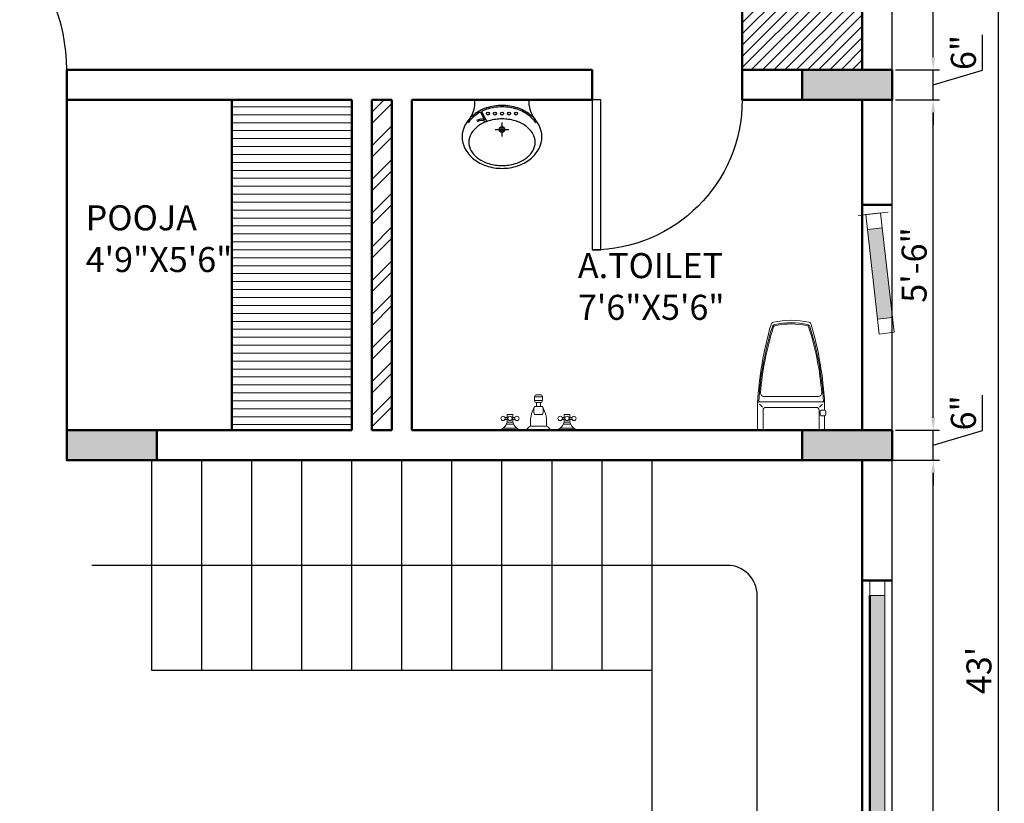
# Model space of a CAD drawing. Units: inches. Extents: x 3064 to 19385, y 846 to 15425.
# Tile 59 of 108: x 6210 to 6407, y 1703 to 1860. Entities that reach past the tile are written whole.
import ezdxf

# ---------------------------------------------------------------- set-up
doc = ezdxf.new("R2010")
doc.units = ezdxf.units.IN
for name, color, linetype, lineweight in [('A-ANNO-DIMS', 2, 'Continuous', 18), ('A-AREA-IDEN', 3, 'Continuous', 18), ('A-COLS', 1, 'Continuous', 35), ('A-DOOR', 3, 'Continuous', 25), ('A-FLOR-FIXT', 9, 'Continuous', 18), ('A-FLOR-STRS', 2, 'Continuous', 25), ('A-FURN-PATT', 252, 'Continuous', 13), ('A-GLAZ', 4, 'Continuous', 18), ('A-WALL', 7, 'Continuous', 50), ('C-PROP', 6, 'Continuous', 25)]:
    doc.layers.add(name, color=color, linetype=linetype, lineweight=lineweight)
doc.layers.add('THIET-BI', color=21, linetype='Continuous')
doc.styles.get("Standard").update_dxf_attribs({"font": 'arial.ttf'})
doc.dimstyles.new('ISO-25', dxfattribs={"dimtxt": 9, "dimasz": 2.5, "dimexe": 1.25, "dimexo": 0.625, "dimtad": 1, "dimdec": 1, "dimlunit": 3, "dimtxsty": 'Standard', "dimcen": 2.5, "dimadec": 0, "dimazin": 0, "dimtfac": 1, "dimtdec": 1, "dimtmove": 0, "dimatfit": 3, "dimfxl": 1, "dimarcsym": 0})

# ---------------------------------------------------------------- blocks, each defined once
blk = doc.blocks.new('*U3')
for p, q in [((0, 0), (0, -6)), ((36, 0), (36, -6))]:
    blk.add_line(p, q)
blk.add_lwpolyline([(0, 0), (0, 36), (1.75, 36), (1.75, 0)], close=True)
blk.add_arc((0, 0), 36, 0, 90)
blk = doc.blocks.new('*U4')
for p, q in [((0, 0), (0, -6)), ((30, 0), (30, -6))]:
    blk.add_line(p, q)
blk.add_lwpolyline([(0, 0), (0, 30), (1.75, 30), (1.75, 0)], close=True)
blk.add_arc((0, 0), 30, 0, 90)
blk = doc.blocks.new('A$C430D11A0')
at = {"layer": 'THIET-BI'}
for p, q in [((90, 445), (90, 485)), ((475, 485), (90, 485)), ((475, 483), (90, 483)), ((475, 445), (475, 485)), ((129.4, 398.5), (158.2, 344.4)), ((138.3, 403), (176, 332.4)), ((282.5, 226.2), (282.5, 324.8)), ((233.4, 275.5), (331.9, 275.5))]:
    blk.add_line(p, q, dxfattribs=at)
for points in [[(565, 222.5, 0.121635), (544.7, 304.8, 0.10526), (482.3, 379.8, 0.088175), (393.4, 427.4, 0.079002), (282.5, 445, 0.079002), (171.6, 427.4, 0.088175), (82.7, 379.8, 0.10526), (20.3, 304.8, 0.121635), (0, 222.5, 0.121635), (20.3, 140.2, 0.10526), (82.7, 65.2, 0.088175), (171.6, 17.6, 0.079002), (282.5, 0, 0.079002), (393.4, 17.6, 0.088175), (482.3, 65.2, 0.10526), (544.7, 140.2, 0.121635)], [(517.5, 185, 0.134042), (501.2, 244.9, 0.106817), (448.7, 301.7, 0.082468), (375.6, 336.7, 0.070874), (282.5, 350, 0.070874), (189.4, 336.7, 0.082468), (116.3, 301.7, 0.106817), (63.8, 244.9, 0.134042), (47.5, 185, 0.134042), (63.8, 125.1, 0.106817), (116.3, 68.3, 0.082468), (189.4, 33.3, 0.070874), (282.5, 20, 0.070874), (375.6, 33.3, 0.082468), (448.7, 68.3, 0.106817), (501.2, 125.1, 0.134042)]]:
    blk.add_lwpolyline(points, format="xyb", close=True, dxfattribs=at)
for points in [[(522.9, 321.6, 0.07708), (476.1, 372, 0.088175), (390.3, 417.9, 0.079002), (282.5, 435, 0.079002), (174.7, 417.9, 0.035427), (138.3, 403, 0.07708)], [(129.4, 398.5, 0.043566), (88.9, 372, 0.07708), (42.1, 321.6, 0.041486)]]:
    blk.add_lwpolyline(points, format="xyb", dxfattribs=at)
for centre, radius in [((182.5, 388.2), 10.5), ((232.5, 388.2), 10.5), ((282.5, 388.2), 10.5), ((332.5, 388.2), 10.5), ((382.5, 388.2), 10.5), ((282.5, 275.5), 20), ((282.5, 275.5), 15)]:
    blk.add_circle(centre, radius, dxfattribs=at)
for centre, radius, start, end in [((-103.8, 468.9), 195.3, 320.8253, 352.95569), ((668.8, 468.9), 195.3, 187.04431, 219.1747), ((136.4, 285.4), 62.9, 69.64296, 123.47738), ((136.4, 285.4), 52.9, 55.24551, 123.47738)]:
    blk.add_arc(centre, radius, start, end, dxfattribs=at)
blk = doc.blocks.new('WC-P05')
for p, q in [((-202.4, 531.6), (-202.4, 439.1)), ((-192.4, 541.6), (262.6, 541.6)), ((-163.4, 541.6), (-163.4, 400.6)), ((233.6, 541.6), (233.6, 400.6)), ((272.6, 531.6), (272.6, 351.6)), ((-210.4, 430.1), (-210.4, 409.1)), ((-201.4, 439.1), (-180.4, 439.1)), ((-171.4, 430.1), (-171.4, 409.1)), ((-202.4, 400.1), (-202.4, 351.6)), ((-201.4, 400.1), (-180.4, 400.1)), ((-166.9, 378.6), (-188.2, 357.3)), ((-143.4, 380.6), (213.6, 380.6)), ((237.1, 378.6), (258.4, 357.3)), ((-192.4, 341.6), (262.6, 341.6)), ((-159.3, 302.6), (229.5, 302.6))]:
    blk.add_line(p, q)
blk.add_lwpolyline([(-90.9, -221.9, 0.114547), (161, -222, 0.114547)], format="xyb")
for centre, radius, start, end in [((-192.4, 531.6), 10, 90, 180), ((262.6, 531.6), 10, 0, 90), ((-201.4, 430.1), 9, 90, 180), ((-180.4, 430.1), 9, 0, 90), ((-201.4, 409.1), 9, 180, 270), ((2308.9, 492.3), 2515.2, 183.20675, 196.12415), ((-192.4, 351.6), 10, 180, 270), ((-180.4, 409.1), 9, 270, 0), ((-143.4, 400.6), 20, 180, 270), ((-2238.7, 492.3), 2515.2, 343.87268, 356.79325), ((213.6, 400.6), 20, 270, 0), ((262.6, 351.6), 10, 270, 0), ((1906, 447.2), 2102.6, 182.87428, 197.65536), ((-159.3, 280.1), 22.5, 90, 184.62462), ((-1835.8, 447.2), 2102.6, 342.34464, 357.12572), ((229.5, 280.1), 22.5, 355.37538, 90), ((1905.9, 447.2), 2094.5, 184.62454, 197.52765), ((-1835.8, 447.2), 2094.6, 342.46396, 355.37538), ((-85.8, -199.9), 22.5, 196.12415, 256.89941), ((-76.1, -183.7), 22.5, 197.65536, 257.50587), ((-69.9, -176.8), 22.5, 197.52765, 258.10049), ((35.1, 318), 536.4, 257.50587, 282.49413), ((35.7, 324.3), 534.7, 258.10049, 281.73735), ((139.9, -177.1), 22.5, 281.73735, 342.46396), ((146.2, -183.7), 22.5, 282.49413, 342.34464), ((155.9, -200.1), 22.5, 283.03778, 343.87268)]:
    blk.add_arc(centre, radius, start, end)
blk = doc.blocks.new('Faucet - Bathroom front')
for p, q in [((-0.5, 4.25), (0.5, 4.25)), ((0.5, 3.75), (-0.5, 3.75)), ((-0.5, 3), (0.5, 3)), ((-0.25, 3), (-0.25, 3.5)), ((0.25, 3.5), (0.25, 3)), ((-4, 1.625), (-4.25, 1.625)), ((-4, 1.375), (-4.25, 1.375)), ((-3.25, 1.625), (-3, 1.625)), ((-3.25, 1.375), (-3, 1.375)), ((0.5, 2), (-0.5, 2)), ((3.25, 1.625), (3, 1.625)), ((3.25, 1.375), (3, 1.375)), ((4, 1.625), (4.25, 1.625)), ((4, 1.375), (4.25, 1.375)), ((-5, 0), (-2.25, 0)), ((-4.5087, 0.25), (-2.7408, 0.25)), ((-3.1442, 0.75), (-4.0979, 0.75)), ((-1.5, 0), (1.5, 0)), ((-1, 0.5), (1, 0.5)), ((2.25, 0), (5, 0)), ((2.7413, 0.25), (4.5092, 0.25)), ((4.1058, 0.75), (3.1521, 0.75))]:
    blk.add_line(p, q)
for points in [[(-0.5, 3.75), (-0.5, 4.25)], [(-0.25, 4.5), (0.25, 4.5)], [(0.5, 4.25), (0.5, 3.75)], [(0.25, 3.5), (-0.25, 3.5)]]:
    blk.add_lwpolyline(points)
for points in [[(-4, 1), (-4, 2), (-3.25, 2), (-3.25, 1)], [(3.25, 1), (3.25, 2), (4, 2), (4, 1)]]:
    blk.add_lwpolyline(points, close=True)
for centre in [(-4.5, 1.5), (-3.625, 1.5), (-2.75, 1.5), (2.75, 1.5), (3.625, 1.5), (4.5, 1.5)]:
    blk.add_circle(centre, 0.2795)
for centre, radius, start, end in [((-0.2575, 4.2575), 0.2426, 88.22243, 181.7776), ((0.2575, 4.2575), 0.2426, 358.2224, 91.77757), ((3, 1), 4.0311, 150.2551, 187.125), ((0.6413, 2.5), 1.246, 156.3417, 203.6583), ((-0.2575, 3.7425), 0.2426, 178.2224, 271.7776), ((0.2575, 3.7425), 0.2426, 268.2224, 1.777565), ((-3, 1), 4.0311, 352.875, 29.74488), ((-0.6413, 2.5), 1.246, 336.3417, 23.65835), ((-5.375, 1.375), 1.4252, 285.2551, 344.7449), ((-1.875, 1.375), 1.4252, 195.2551, 254.7449), ((-0.7962, -0.2038), 0.7327, 106.1502, 163.8498), ((0.7962, -0.2038), 0.7327, 16.1502, 73.84979), ((1.875, 1.375), 1.4252, 285.2551, 344.7449), ((5.375, 1.375), 1.4252, 195.2551, 254.7449)]:
    blk.add_arc(centre, radius, start, end)
blk = doc.blocks.new('*D350')
at = {"layer": 'A-ANNO-DIMS', "color": 0, "lineweight": -2, "transparency": 16777216}
for p, q in [((6379.12, 1771.99), (6393.94, 1771.99)), ((6392.69, 1576.49), (6392.69, 1769.49)), ((6379.12, 1573.99), (6393.94, 1573.99))]:
    blk.add_line(p, q, dxfattribs=at)
at = {"layer": 'A-ANNO-DIMS', "color": 0, "transparency": 16777216}
for points in [[(6392.27, 1769.49), (6393.1, 1769.49), (6392.69, 1771.99)], [(6392.27, 1576.49), (6393.1, 1576.49), (6392.69, 1573.99)]]:
    blk.add_solid(points, dxfattribs=at)
at = {"layer": 'Defpoints', "color": 0, "transparency": 16777216}
for p in [(6378.49, 1771.99), (6392.69, 1771.99), (6378.49, 1573.99)]:
    blk.add_point(p, dxfattribs=at)
at = {"layer": 'A-ANNO-DIMS', "color": 0, "transparency": 16777216, "insert": (6389.51, 1672.99), "char_height": 5, "attachment_point": 5, "rotation": 90}
blk.add_mtext('16\'-6"', dxfattribs=at)
blk = doc.blocks.new('*D351')
at = {"layer": 'A-ANNO-DIMS', "color": 0, "lineweight": -2, "transparency": 16777216}
for p, q in [((6402.53, 1777.94), (6402.53, 1784.97)), ((6392.69, 1780.49), (6392.69, 1782.99)), ((6385.12, 1777.99), (6393.94, 1777.99)), ((6392.69, 1771.99), (6392.69, 1777.99)), ((6392.69, 1771.99), (6392.69, 1777.99)), ((6392.69, 1774.99), (6402.53, 1777.94)), ((6379.12, 1771.99), (6393.94, 1771.99)), ((6392.69, 1769.49), (6392.69, 1766.99))]:
    blk.add_line(p, q, dxfattribs=at)
at = {"layer": 'A-ANNO-DIMS', "color": 0, "transparency": 16777216}
for points in [[(6392.27, 1780.49), (6393.1, 1780.49), (6392.69, 1777.99)], [(6392.27, 1769.49), (6393.1, 1769.49), (6392.69, 1771.99)]]:
    blk.add_solid(points, dxfattribs=at)
at = {"layer": 'Defpoints', "color": 0, "transparency": 16777216}
for p in [(6384.49, 1777.99), (6392.69, 1777.99), (6378.49, 1771.99)]:
    blk.add_point(p, dxfattribs=at)
at = {"layer": 'A-ANNO-DIMS', "color": 0, "transparency": 16777216, "insert": (6399.35, 1781.45), "char_height": 5, "attachment_point": 5, "rotation": 90}
blk.add_mtext('6"', dxfattribs=at)
blk = doc.blocks.new('*D352')
at = {"layer": 'A-ANNO-DIMS', "color": 0, "lineweight": -2, "transparency": 16777216}
for p, q in [((6385.12, 1843.99), (6393.94, 1843.99)), ((6392.69, 1780.49), (6392.69, 1841.49)), ((6385.12, 1777.99), (6393.94, 1777.99))]:
    blk.add_line(p, q, dxfattribs=at)
at = {"layer": 'A-ANNO-DIMS', "color": 0, "transparency": 16777216}
for points in [[(6392.27, 1841.49), (6393.1, 1841.49), (6392.69, 1843.99)], [(6392.27, 1780.49), (6393.1, 1780.49), (6392.69, 1777.99)]]:
    blk.add_solid(points, dxfattribs=at)
at = {"layer": 'Defpoints', "color": 0, "transparency": 16777216}
for p in [(6384.49, 1843.99), (6392.69, 1843.99), (6384.49, 1777.99)]:
    blk.add_point(p, dxfattribs=at)
at = {"layer": 'A-ANNO-DIMS', "color": 0, "transparency": 16777216, "insert": (6389.51, 1810.99), "char_height": 5, "attachment_point": 5, "rotation": 90}
blk.add_mtext('5\'-6"', dxfattribs=at)
blk = doc.blocks.new('*D353')
at = {"layer": 'A-ANNO-DIMS', "color": 0, "lineweight": -2, "transparency": 16777216}
for p, q in [((6402.53, 1849.94), (6402.53, 1856.97)), ((6392.69, 1852.49), (6392.69, 1854.99)), ((6385.12, 1849.99), (6393.94, 1849.99)), ((6392.69, 1843.99), (6392.69, 1849.99)), ((6392.69, 1843.99), (6392.69, 1849.99)), ((6392.69, 1846.99), (6402.53, 1849.94)), ((6385.12, 1843.99), (6393.94, 1843.99)), ((6392.69, 1841.49), (6392.69, 1838.99))]:
    blk.add_line(p, q, dxfattribs=at)
at = {"layer": 'A-ANNO-DIMS', "color": 0, "transparency": 16777216}
for points in [[(6392.27, 1852.49), (6393.1, 1852.49), (6392.69, 1849.99)], [(6392.27, 1841.49), (6393.1, 1841.49), (6392.69, 1843.99)]]:
    blk.add_solid(points, dxfattribs=at)
at = {"layer": 'Defpoints', "color": 0, "transparency": 16777216}
for p in [(6384.49, 1849.99), (6392.69, 1849.99), (6384.49, 1843.99)]:
    blk.add_point(p, dxfattribs=at)
at = {"layer": 'A-ANNO-DIMS', "color": 0, "transparency": 16777216, "insert": (6399.35, 1853.45), "char_height": 5, "attachment_point": 5, "rotation": 90}
blk.add_mtext('6"', dxfattribs=at)
blk = doc.blocks.new('*D375')
at = {"layer": 'A-ANNO-DIMS', "color": 0, "lineweight": -2, "transparency": 16777216}
for p, q in [((6379.12, 1981.99), (6393.94, 1981.99)), ((6392.69, 1852.49), (6392.69, 1979.49)), ((6385.12, 1849.99), (6393.94, 1849.99))]:
    blk.add_line(p, q, dxfattribs=at)
at = {"layer": 'A-ANNO-DIMS', "color": 0, "transparency": 16777216}
for points in [[(6392.27, 1979.49), (6393.1, 1979.49), (6392.69, 1981.99)], [(6392.27, 1852.49), (6393.1, 1852.49), (6392.69, 1849.99)]]:
    blk.add_solid(points, dxfattribs=at)
at = {"layer": 'Defpoints', "color": 0, "transparency": 16777216}
for p in [(6378.49, 1981.99), (6392.69, 1981.99), (6384.49, 1849.99)]:
    blk.add_point(p, dxfattribs=at)
at = {"layer": 'A-ANNO-DIMS', "color": 0, "transparency": 16777216, "insert": (6389.55, 1915.99), "char_height": 5, "attachment_point": 5, "rotation": 90}
blk.add_mtext("11'", dxfattribs=at)
blk = doc.blocks.new('*D377')
at = {"layer": 'A-ANNO-DIMS', "color": 0, "lineweight": -2, "transparency": 16777216}
for p, q in [((6385.12, 1987.99), (6406.89, 1987.99)), ((6405.64, 1985.49), (6405.64, 1474.49)), ((6385.12, 1471.99), (6406.89, 1471.99))]:
    blk.add_line(p, q, dxfattribs=at)
at = {"layer": 'A-ANNO-DIMS', "color": 0, "transparency": 16777216}
for points in [[(6405.22, 1985.49), (6406.05, 1985.49), (6405.64, 1987.99)], [(6405.22, 1474.49), (6406.05, 1474.49), (6405.64, 1471.99)]]:
    blk.add_solid(points, dxfattribs=at)
at = {"layer": 'Defpoints', "color": 0, "transparency": 16777216}
for p in [(6384.49, 1987.99), (6384.49, 1471.99), (6405.64, 1471.99)]:
    blk.add_point(p, dxfattribs=at)
at = {"layer": 'A-ANNO-DIMS', "color": 0, "transparency": 16777216, "insert": (6402.46, 1729.99), "char_height": 5, "attachment_point": 5, "rotation": 90}
blk.add_mtext("43'", dxfattribs=at)
blk = doc.blocks.new('WIN-1800-PAIR')
h = blk.add_hatch(color=256)
h.dxf.hatch_style = 1
h.paths.add_polyline_path([(0, 0), (3, 0), (3, 70.5), (0, 70.5)])
h.paths.add_polyline_path([(3, 144), (0, 144), (0, 73.5), (3, 73.5)])
blk.add_line((3, 144), (3, 73.5))
blk.add_lwpolyline([(3, 144), (0, 144), (0, 147), (3, 147)], close=True)
blk = doc.blocks.new('WIN-600-B')
h = blk.add_hatch(color=256)
h.dxf.hatch_style = 1
h.paths.add_polyline_path([(4.5, 21), (1.5, 21), (1.5, 3), (4.5, 3)])
for p, q in [((1.5, 21), (1.5, 3)), ((4.5, 21), (4.5, 3)), ((0, 0), (6, 0))]:
    blk.add_line(p, q)
for points in [[(4.5, 21), (1.5, 21), (1.5, 24), (4.5, 24)], [(4.5, 0), (1.5, 0), (1.5, 3), (4.5, 3)]]:
    blk.add_lwpolyline(points, close=True)

msp = doc.modelspace()

# ---------------------------------------------------------------- hatches: boundary and pattern name
at = {"layer": 'A-COLS'}
h = msp.add_hatch(color=256, dxfattribs=at)
h.dxf.hatch_style = 1
h.paths.add_polyline_path([(6384.49, 1843.99), (6384.49, 1849.99), (6366.49, 1849.99), (6366.49, 1843.99)])
h = msp.add_hatch(color=256, dxfattribs=at)
h.dxf.hatch_style = 1
h.paths.add_polyline_path([(6237.49, 1771.99), (6237.49, 1777.99), (6219.49, 1777.99), (6219.49, 1771.99)])
h = msp.add_hatch(color=256, dxfattribs=at)
h.dxf.hatch_style = 1
h.paths.add_polyline_path([(6384.49, 1771.99), (6384.49, 1777.99), (6366.49, 1777.99), (6366.49, 1771.99)])
at = {"layer": 'A-FURN-PATT'}
h = msp.add_hatch(dxfattribs=at)
h.set_pattern_fill('ANSI31', color=256, scale=0.5)
h.set_pattern_definition([(45, (726.825, 591.649), (-1.122532, 1.122532), [])])
h.paths.add_polyline_path([(6354.49, 1849.99), (6378.49, 1849.99), (6378.49, 1981.99), (6354.49, 1981.99)])
h = msp.add_hatch(dxfattribs=at)
h.set_pattern_fill('ANSI31', color=256, scale=0.5, angle=135)
h.set_pattern_definition([(180, (726.825, 591.649), (-1e-16, -1.5875), [])])
h.paths.add_polyline_path([(6252.49, 1777.99), (6276.49, 1777.99), (6276.49, 1843.99), (6252.49, 1843.99)])
h = msp.add_hatch(dxfattribs=at)
h.set_pattern_fill('ANSI32', color=256, scale=0.5)
h.set_pattern_definition([(45, (726.825, 591.649), (-3.367596, 3.367596), []), (45, (729.07, 591.649), (-3.367596, 3.367596), [])])
h.paths.add_polyline_path([(6280.49, 1777.99), (6284.49, 1777.99), (6284.49, 1843.99), (6280.49, 1843.99)])

# ---------------------------------------------------------------- linework, layer by layer
at = {"layer": 'A-FLOR-STRS'}
for p, q in [((6236.49, 1729.99), (6236.49, 1771.99)), ((6246.49, 1729.99), (6246.49, 1771.99)), ((6256.49, 1729.99), (6256.49, 1771.99)), ((6266.49, 1729.99), (6266.49, 1771.99)), ((6276.49, 1729.99), (6276.49, 1771.99)), ((6286.49, 1729.99), (6286.49, 1771.99)), ((6296.49, 1729.99), (6296.49, 1771.99)), ((6306.49, 1729.99), (6306.49, 1771.99)), ((6316.49, 1729.99), (6316.49, 1771.99)), ((6326.49, 1729.99), (6326.49, 1771.99)), ((6336.49, 1615.99), (6336.49, 1771.99)), ((6336.49, 1729.99), (6236.49, 1729.99))]:
    msp.add_line(p, q, dxfattribs=at)
msp.add_lwpolyline([(6243.98, 1594.99), (6351.49, 1594.99, 0.414214), (6357.49, 1600.99), (6357.49, 1744.99, 0.414214), (6351.49, 1750.99), (6224.49, 1750.99)], format="xyb", dxfattribs=at)
at = {"layer": 'A-WALL'}
for p, q in [((6354.49, 1843.99), (6354.49, 1981.99)), ((6378.49, 1849.99), (6378.49, 1981.99)), ((6324.49, 1849.99), (6219.49, 1849.99)), ((6219.49, 1849.99), (6219.49, 1771.99)), ((6324.49, 1843.99), (6324.49, 1849.99)), ((6378.49, 1849.99), (6354.49, 1849.99)), ((6276.49, 1843.99), (6219.49, 1843.99)), ((6252.49, 1843.99), (6252.49, 1777.99)), ((6276.49, 1843.99), (6276.49, 1777.99)), ((6284.49, 1843.99), (6280.49, 1843.99)), ((6280.49, 1843.99), (6280.49, 1777.99)), ((6284.49, 1777.99), (6284.49, 1843.99)), ((6288.49, 1777.99), (6288.49, 1843.99)), ((6324.49, 1843.99), (6288.49, 1843.99)), ((6378.49, 1843.99), (6354.49, 1843.99)), ((6378.49, 1777.99), (6378.49, 1843.99)), ((6378.49, 1822.99), (6384.49, 1822.99)), ((6276.49, 1777.99), (6219.49, 1777.99)), ((6284.49, 1777.99), (6280.49, 1777.99)), ((6378.49, 1777.99), (6288.49, 1777.99)), ((6378.49, 1771.99), (6219.49, 1771.99)), ((6378.49, 1573.99), (6378.49, 1771.99)), ((6384.49, 1747.99), (6378.49, 1747.99)), ((6379.99, 1744.99), (6379.99, 1674.49))]:
    msp.add_line(p, q, dxfattribs=at)
for points in [[(6384.49, 1849.99), (6366.49, 1849.99), (6366.49, 1843.99), (6384.49, 1843.99)], [(6237.49, 1777.99), (6219.49, 1777.99), (6219.49, 1771.99), (6237.49, 1771.99)], [(6384.49, 1777.99), (6366.49, 1777.99), (6366.49, 1771.99), (6384.49, 1771.99)]]:
    msp.add_lwpolyline(points, close=True, dxfattribs=at)
at = {"layer": 'C-PROP'}
msp.add_line((6384.49, 1471.99), (6384.49, 1987.99), dxfattribs=at)

# ---------------------------------------------------------------- block references
at = {"layer": 'A-DOOR'}
msp.add_blockref('*U3', (6183.49, 1849.99), dxfattribs=at)
at = {"layer": 'A-DOOR', "xscale": -1, "rotation": 180}
msp.add_blockref('*U4', (6324.49, 1843.99), dxfattribs=at)
at = {"layer": 'A-FLOR-FIXT'}
for name, p, xscale, yscale, zscale in [('A$C430D11A0', (6298.52, 1830.3), 0.0282220760332506, 0.0282220760332506, 0.0282220760332506), ('Faucet - Bathroom front', (6313.79, 1777.99), 1.573166238287219, 1.573166238287219, 1.573166238287219)]:
    msp.add_blockref(name, p, dxfattribs=dict(at, xscale=xscale, yscale=yscale, zscale=zscale))
at = {"layer": 'A-FLOR-FIXT', "xscale": 0.0282220760332506, "yscale": 0.0282220760332506, "zscale": 0.0282220760332506, "rotation": 180}
msp.add_blockref('WC-P05', (6365.27, 1793.28), dxfattribs=at)
at = {"layer": 'A-GLAZ', "rotation": 186.4416000993554}
msp.add_blockref('WIN-600-B', (6383.65, 1821.56), dxfattribs=at)
at = {"layer": 'A-GLAZ'}
msp.add_blockref('WIN-1800-PAIR', (6379.99, 1600.99), dxfattribs=at)

# ---------------------------------------------------------------- texts
at = {"layer": 'A-AREA-IDEN', "char_height": 5, "attachment_point": 1}
for s, insert in [('POOJA\\P4\'9"X5\'6"', (6223.28, 1822.92)), ('A.TOILET\\P7\'6"X5\'6"', (6321.66, 1813.37))]:
    msp.add_mtext_dynamic_manual_height_columns(s, width=67.5924, gutter_width=12.5, heights=[0], dxfattribs=dict(at, insert=insert))

# ---------------------------------------------------------------- dimensions: what is measured, and where the dimension line sits
at = {"layer": 'A-ANNO-DIMS'}
for base, p1, p2, override, picture, middle in [((6405.64, 1471.99), (6384.49, 1987.99), (6384.49, 1471.99), {"dimtxt": 5, "dimclrd": 0, "dimclre": 0, "dimclrt": 0}, '*D377', (6402.46, 1729.99)), ((6392.69, 1981.99), (6384.49, 1849.99), (6378.49, 1981.99), {"dimtxt": 5, "dimclrd": 0, "dimclre": 0, "dimclrt": 0, "dimtmove": 1}, '*D375', (6389.55, 1915.99)), ((6392.69, 1849.99), (6384.49, 1843.99), (6384.49, 1849.99), {"dimtxt": 5, "dimclrd": 0, "dimclre": 0, "dimclrt": 0, "dimtmove": 1}, '*D353', (6399.35, 1850.57)), ((6392.69, 1843.99), (6384.49, 1777.99), (6384.49, 1843.99), {"dimtxt": 5, "dimclrd": 0, "dimclre": 0, "dimclrt": 0, "dimtmove": 1}, '*D352', (6389.51, 1810.99)), ((6392.69, 1777.99), (6378.49, 1771.99), (6384.49, 1777.99), {"dimtxt": 5, "dimclrd": 0, "dimclre": 0, "dimclrt": 0, "dimtmove": 1}, '*D351', (6399.35, 1778.57)), ((6392.69, 1771.99), (6378.49, 1573.99), (6378.49, 1771.99), {"dimtxt": 5, "dimclrd": 0, "dimclre": 0, "dimclrt": 0, "dimtmove": 1}, '*D350', (6389.51, 1672.99))]:
    dim = msp.add_linear_dim(base=base, p1=p1, p2=p2, angle=90, dimstyle='ISO-25', override=override, dxfattribs=at)
    dim.commit()
    dim.dimension.update_dxf_attribs({"geometry": picture, "text_midpoint": middle})

doc.saveas('drawing.dxf')
